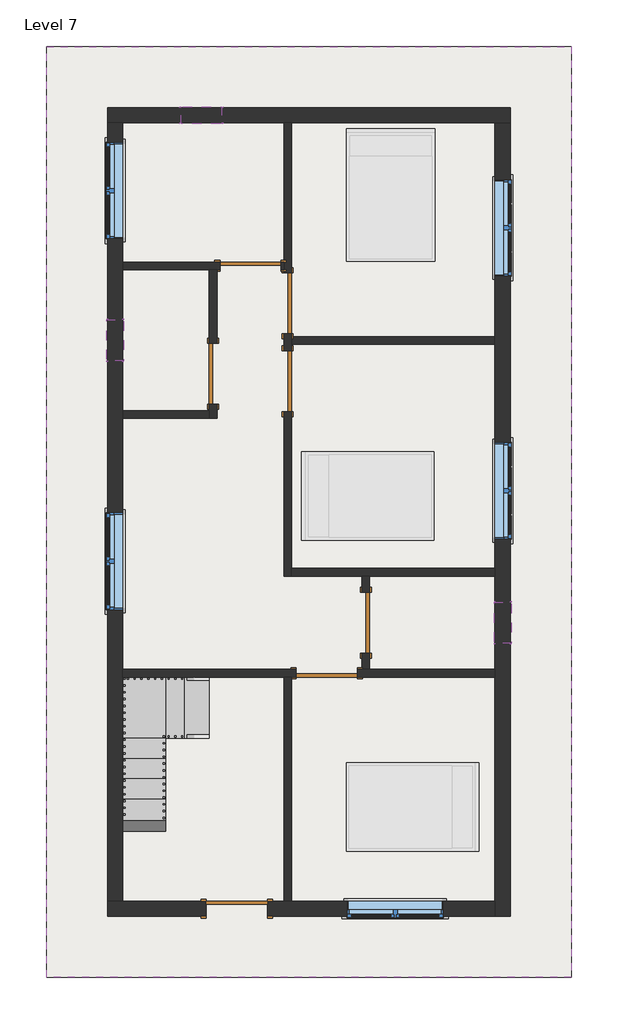
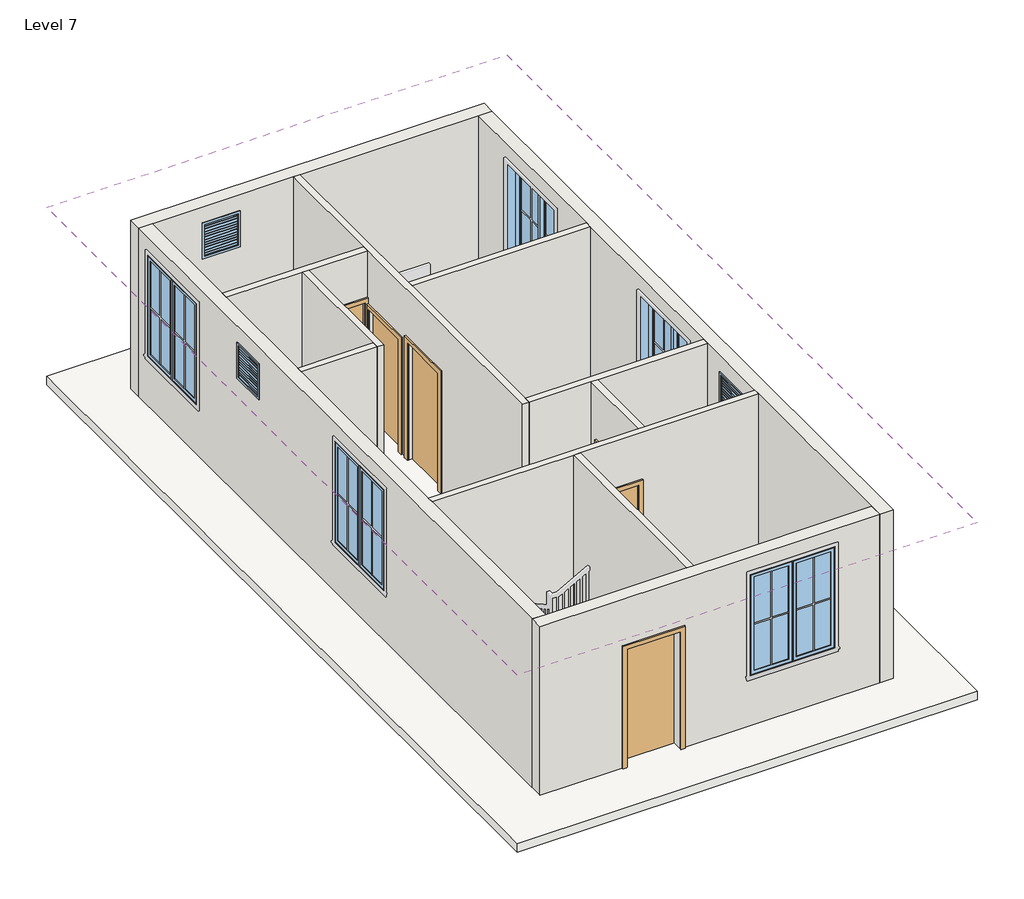
# One storey, part 1 of 2: 13 walls, 8 windows, 7 doors, 2 roofs, 1 stair flight.
"""IFC4 building model written with IfcOpenShell, lengths in millimetres."""

from ifc_helpers import new_model, si_unit, frame, origin, place, context, project, spatial, polyline, outline, extrude, faceted_brep, transform, mapped, element, save
from components import door_5e62189b, door_17d80c48, door_e5f9f3c4, door_305aa2a5, door_0ca8825f, window_9ac97e1a, window_f2d8fef0

model = new_model("IFC4")

# Units and contexts
model_context = context("Model", 3, world=origin())
ifc_project = project(units=[si_unit("LENGTHUNIT", "METRE", prefix="MILLI")], contexts=[model_context])

# Site, building, storey
site = spatial("IfcSite", under=ifc_project)
building = spatial("IfcBuilding", under=site)
storey = spatial("IfcBuildingStorey", under=building, Name="Level 7", Elevation=16002.0)

# Doors
placement = place(None, origin())
door_shape = door_5e62189b(model_context)
element("IfcDoor", 1, ObjectType="Single-Flush : 36\" x 80\"", at=placement, inside=storey, context=model_context, shape_type="MappedRepresentation", body=[
    mapped(door_shape, transform((-2690.3389285, 2204.6069249, 16002.0), x_axis=(0.0, -1.0, 0.0), y_axis=(1.0, 0.0, 0.0), z_axis=(0.0, 0.0, 1.0))),
])
element("IfcDoor", 2, ObjectType="Single-Flush : 36\" x 80\"", at=placement, inside=storey, context=model_context, shape_type="MappedRepresentation", body=[
    mapped(door_shape, transform((-404.3389285, -1522.8430751, 16002.0), x_axis=(0.0, 1.0, 0.0), y_axis=(-1.0, 0.0, 0.0), z_axis=(0.0, 0.0, 1.0))),
])
door_2_shape = door_17d80c48(model_context)
element("IfcDoor", 3, ObjectType="Single-Flush : 36\" x 80\"", at=placement, inside=storey, context=model_context, shape_type="MappedRepresentation", body=[
    mapped(door_2_shape, transform((-1572.7389285, 3258.7069249, 16002.0), x_axis=(0.0, -1.0, 0.0), y_axis=(1.0, 0.0, 0.0), z_axis=(0.0, 0.0, 1.0))),
])
door_3_shape = door_e5f9f3c4(model_context)
element("IfcDoor", 4, ObjectType="Single-Flush : 36\" x 84\"", at=placement, inside=storey, context=model_context, shape_type="MappedRepresentation", body=[
    mapped(door_3_shape, transform((-2131.5389285, 3817.5069249, 16002.0), x_axis=(1.0, 0.0, 0.0), y_axis=(0.0, 1.0, 0.0), z_axis=(0.0, 0.0, 1.0))),
])
element("IfcDoor", 5, ObjectType="Single-Flush : 36\" x 84\"", at=placement, inside=storey, context=model_context, shape_type="MappedRepresentation", body=[
    mapped(door_3_shape, transform((-988.5389285, -2278.4930751, 16002.0), x_axis=(-1.0, 0.0, 0.0), y_axis=(0.0, -1.0, 0.0), z_axis=(0.0, 0.0, 1.0))),
])
door_4_shape = door_305aa2a5(model_context)
element("IfcDoor", 6, ObjectType="Single-Flush : 36\" x 84\"", at=placement, inside=storey, context=model_context, shape_type="MappedRepresentation", body=[
    mapped(door_4_shape, transform((-1572.7389285, 2090.3069249, 16002.0), x_axis=(0.0, 1.0, 0.0), y_axis=(-1.0, 0.0, 0.0), z_axis=(0.0, 0.0, 1.0))),
])
door_5_shape = door_0ca8825f(model_context)
element("IfcDoor", 7, ObjectType="Single-Flush : 36\" x 84\"", at=placement, inside=storey, context=model_context, shape_type="MappedRepresentation", body=[
    mapped(door_5_shape, transform((-2334.7389285, -5802.7430751, 16002.0), x_axis=(1.0, 0.0, 0.0), y_axis=(0.0, 1.0, 0.0), z_axis=(0.0, 0.0, 1.0))),
])

# Roofs
element("IfcRoof", 8, ObjectType="ROOF 6\"", at=placement, inside=storey, context=model_context, shape_type="SweptSolid", body=[
    extrude(outline(polyline([(-5185.8889285, 7100.4569249), (2675.4110715, 7100.4569249), (2675.4110715, -6831.4430751), (-5185.8889285, -6831.4430751), (-5185.8889285, 7100.4569249)])), frame((0.0, 0.0, 15849.6), z_axis=(0.0, 0.0, 1.0), x_axis=(1.0, 0.0, 0.0)), (0.0, 0.0, 1.0), 152.4),
])
element("IfcRoof", 9, ObjectType="ROOF 6\"", at=placement, inside=storey, context=model_context, shape_type="SweptSolid", body=[
    extrude(outline(polyline([(-5185.8889285, 7100.4569249), (2675.4110715, 7100.4569249), (2675.4110715, -6831.4430751), (-5185.8889285, -6831.4430751), (-5185.8889285, 7100.4569249)])), frame((0.0, 0.0, 19050.0), z_axis=(0.0, 0.0, 1.0), x_axis=(1.0, 0.0, 0.0)), (0.0, 0.0, 1.0), 152.4),
])

# Stair flight
element("IfcStairFlight", 10, ObjectType="3/4\" Nosing", at=placement, inside=storey, context=model_context, shape_type="Brep", body=[
    faceted_brep([(-2747.4889285, -3250.0430751, 16171.3333333), (-2747.4889285, -2335.6430751, 16171.3333333), (-3128.4889285, -2335.6430751, 16171.3333333), (-3128.4889285, -3250.0430751, 16171.3333333), (-3128.4889285, -3250.0430751, 16107.8333333), (-2754.6326785, -3250.0430751, 16107.8333333), (-2754.6326785, -2335.6430751, 16107.8333333), (-3128.4889285, -2335.6430751, 16107.8333333)], [[[0, 1, 2, 3]], [[0, 3, 4, 5]], [[2, 1, 6, 7]], [[1, 0, 5, 6]], [[4, 7, 6, 5]], [[7, 4, 3, 2]]]),
    faceted_brep([(-3128.4889285, -3250.0430751, 16340.6666667), (-3128.4889285, -2335.6430751, 16340.6666667), (-3401.5389285, -2335.6430751, 16340.6666667), (-3401.5389285, -3250.0430751, 16340.6666667), (-3401.5389285, -3250.0430751, 16277.1666667), (-3135.6326785, -3250.0430751, 16277.1666667), (-3135.6326785, -2335.6430751, 16277.1666667), (-3401.5389285, -2335.6430751, 16277.1666667)], [[[0, 1, 2, 3]], [[0, 3, 4, 5]], [[2, 1, 6, 7]], [[1, 0, 5, 6]], [[4, 7, 6, 5]], [[7, 4, 3, 2]]]),
    faceted_brep([(-3401.5389285, -3269.0930751, 16510.0), (-3401.5389285, -3250.0430751, 16510.0), (-3401.5389285, -2335.6430751, 16510.0), (-4042.8889285, -2335.6430751, 16510.0), (-4042.8889285, -3269.0930751, 16510.0), (-3401.5389285, -3269.0930751, 16446.5), (-3401.5389285, -3250.0430751, 16446.5), (-3408.6826785, -3250.0430751, 16446.5), (-3408.6826785, -2335.6430751, 16446.5), (-4042.8889285, -2335.6430751, 16446.5), (-4042.8889285, -3269.0930751, 16446.5), (-3401.5389285, -3250.0430751, 16679.3333333), (-4042.8889285, -3250.0430751, 16679.3333333), (-4042.8889285, -3285.5502386, 16679.3333333), (-4042.8889285, -3573.8930751, 16679.3333333), (-3401.5389285, -3573.8930751, 16679.3333333), (-3401.5389285, -3285.5502386, 16679.3333333), (-3401.5389285, -3573.8930751, 16606.7200976), (-3401.5389285, -3285.5502386, 16446.5), (-4042.8889285, -3285.5502386, 16446.5), (-4042.8889285, -3573.8930751, 16606.7200976), (-3401.5389285, -3554.8430751, 16848.6666667), (-4042.8889285, -3554.8430751, 16848.6666667), (-4042.8889285, -3878.6930751, 16848.6666667), (-3401.5389285, -3878.6930751, 16848.6666667), (-3401.5389285, -3878.6930751, 16776.0847552), (-4042.8889285, -3878.6930751, 16776.0847552), (-3401.5389285, -3859.6430751, 17018.0), (-4042.8889285, -3859.6430751, 17018.0), (-4042.8889285, -4183.4930751, 17018.0), (-3401.5389285, -4183.4930751, 17018.0), (-3401.5389285, -4183.4930751, 16945.4494128), (-4042.8889285, -4183.4930751, 16945.4494128), (-3401.5389285, -4164.4430751, 17187.3333333), (-4042.8889285, -4164.4430751, 17187.3333333), (-4042.8889285, -4488.2930751, 17187.3333333), (-3401.5389285, -4488.2930751, 17187.3333333), (-3401.5389285, -4488.2930751, 17114.8140703), (-4042.8889285, -4488.2930751, 17114.8140703), (-3401.5389285, -4792.8112092, 17356.6666667), (-3401.5389285, -4469.2430751, 17356.6666667), (-4042.8889285, -4469.2430751, 17356.6666667), (-4042.8889285, -4792.8112092, 17356.6666667), (-3401.5389285, -4773.7612092, 17526.0), (-3401.5389285, -5114.0119996, 17526.0), (-3401.5389285, -5114.0119996, 17462.5), (-4042.8889285, -4792.8112092, 17284.0221068), (-4042.8889285, -4773.7612092, 17526.0), (-4042.8889285, -5114.0119996, 17526.0), (-4042.8889285, -5688.4430751, 17526.0), (-3401.5389285, -5688.4430751, 17526.0), (-4042.8889285, -5114.0119996, 17462.5), (-4042.8889285, -5688.4430751, 17462.5), (-3401.5389285, -5688.4430751, 17462.5)], [[[0, 1, 2, 3, 4]], [[1, 0, 5, 6]], [[7, 1, 6]], [[3, 2, 8, 9]], [[4, 3, 9, 10]], [[11, 12, 13, 14, 15, 16]], [[0, 11, 16, 15, 17, 18, 5]], [[12, 4, 10, 19, 20, 14, 13]], [[21, 22, 23, 24]], [[21, 24, 25, 17, 15]], [[23, 22, 14, 20, 26]], [[27, 28, 29, 30]], [[27, 30, 31, 25, 24]], [[29, 28, 23, 26, 32]], [[33, 34, 35, 36]], [[33, 36, 37, 31, 30]], [[35, 34, 29, 32, 38]], [[39, 40, 41, 42]], [[39, 43, 44, 45, 37, 36, 40]], [[42, 41, 35, 38, 46]], [[43, 47, 48, 49, 50, 44]], [[47, 42, 46, 51, 52, 49, 48]], [[50, 49, 52, 53]], [[2, 1, 7, 8]], [[0, 4, 12, 11]], [[15, 14, 22, 21]], [[24, 23, 28, 27]], [[30, 29, 34, 33]], [[36, 35, 41, 40]], [[39, 42, 47, 43]], [[18, 19, 10, 9, 8, 7, 6, 5]], [[19, 18, 17, 25, 31, 37, 45, 51, 46, 38, 32, 26, 20]], [[45, 53, 52, 51]], [[53, 45, 44, 50]]]),
    faceted_brep([(-3401.5389285, -4773.7612092, 17695.3333333), (-3401.5389285, -5688.4430751, 17695.3333333), (-3128.4889285, -5688.4430751, 17695.3333333), (-3128.4889285, -4773.7612092, 17695.3333333), (-3394.3951785, -4773.7612092, 17631.8333333), (-3128.4889285, -4773.7612092, 17631.8333333), (-3394.3951785, -5688.4430751, 17631.8333333), (-3128.4889285, -5688.4430751, 17631.8333333)], [[[0, 1, 2, 3]], [[4, 0, 3, 5]], [[2, 1, 6, 7]], [[1, 0, 4, 6]], [[5, 7, 6, 4]], [[7, 5, 3, 2]]]),
    faceted_brep([(-3128.4889285, -4773.7612092, 17864.6666667), (-3128.4889285, -5688.4430751, 17864.6666667), (-2793.6303845, -5688.4430751, 17864.6666667), (-2793.6303845, -4773.7612092, 17864.6666667), (-2793.6303845, -4773.7612092, 17801.1666667), (-3121.3451785, -4773.7612092, 17801.1666667), (-3121.3451785, -5688.4430751, 17801.1666667), (-2793.6303845, -5688.4430751, 17801.1666667)], [[[0, 1, 2, 3]], [[0, 3, 4, 5]], [[2, 1, 6, 7]], [[3, 2, 7, 4]], [[1, 0, 5, 6]], [[6, 5, 4, 7]]]),
])

# Walls
element("IfcWall", 11, ObjectType="WALL 4.5\"", at=placement, inside=storey, context=model_context, shape_type="Brep", body=[
    faceted_brep([(-1629.8889285, 2801.5069249, 18034.0), (-1629.8889285, 2801.5069249, 16002.0), (-1629.8889285, 2547.5069249, 16002.0), (-1629.8889285, 2547.5069249, 18135.6), (-1629.8889285, 1633.1069249, 18135.6), (-1629.8889285, 1633.1069249, 16002.0), (-1629.8889285, -824.3430751, 16002.0), (-1629.8889285, -824.3430751, 19050.0), (-1629.8889285, 3760.3569249, 19050.0), (-1629.8889285, 3874.6569249, 19050.0), (-1629.8889285, 5957.4569249, 19050.0), (-1629.8889285, 5957.4569249, 16002.0), (-1629.8889285, 3874.6569249, 16002.0), (-1629.8889285, 3760.3569249, 16002.0), (-1629.8889285, 3715.9069249, 16002.0), (-1629.8889285, 3715.9069249, 18034.0), (-1515.5889285, 2547.5069249, 16002.0), (-1515.5889285, 2642.7569249, 16002.0), (-1515.5889285, 2757.0569249, 16002.0), (-1515.5889285, 2801.5069249, 16002.0), (-1515.5889285, 2801.5069249, 18034.0), (-1515.5889285, 3715.9069249, 18034.0), (-1515.5889285, 3715.9069249, 16002.0), (-1515.5889285, 5957.4569249, 16002.0), (-1515.5889285, 5957.4569249, 19050.0), (-1515.5889285, 2757.0569249, 19050.0), (-1515.5889285, 2642.7569249, 19050.0), (-1515.5889285, -710.0430751, 19050.0), (-1515.5889285, -824.3430751, 19050.0), (-1515.5889285, -824.3430751, 16002.0), (-1515.5889285, -710.0430751, 16002.0), (-1515.5889285, 1633.1069249, 16002.0), (-1515.5889285, 1633.1069249, 18135.6), (-1515.5889285, 2547.5069249, 18135.6)], [[[0, 1, 2, 3, 4, 5, 6, 7, 8, 9, 10, 11, 12, 13, 14, 15]], [[16, 17, 18, 19, 20, 21, 22, 23, 24, 25, 26, 27, 28, 29, 30, 31, 32, 33]], [[31, 30, 29, 6, 5]], [[2, 1, 19, 18, 17, 16]], [[14, 13, 12, 11, 23, 22]], [[11, 10, 24, 23]], [[3, 2, 16, 33]], [[4, 3, 33, 32]], [[5, 4, 32, 31]], [[20, 19, 1, 0]], [[21, 20, 0, 15]], [[22, 21, 15, 14]], [[10, 9, 8, 7, 28, 27, 26, 25, 24]], [[7, 6, 29, 28]]]),
])
element("IfcWall", 12, ObjectType="WALL 4.5\"", at=placement, inside=storey, context=model_context, shape_type="Brep", body=[
    faceted_brep([(1532.4110715, -710.0430751, 16002.0), (-1515.5889285, -710.0430751, 16002.0), (-1515.5889285, -710.0430751, 19050.0), (1532.4110715, -710.0430751, 19050.0), (1532.4110715, -824.3430751, 16002.0), (1532.4110715, -824.3430751, 19050.0), (-347.1889285, -824.3430751, 19050.0), (-461.4889285, -824.3430751, 19050.0), (-1515.5889285, -824.3430751, 19050.0), (-1515.5889285, -824.3430751, 16002.0), (-461.4889285, -824.3430751, 16002.0), (-347.1889285, -824.3430751, 16002.0)], [[[0, 1, 2, 3]], [[4, 5, 6, 7, 8, 9, 10, 11]], [[1, 0, 4, 11, 10, 9]], [[0, 3, 5, 4]], [[3, 2, 8, 7, 6, 5]], [[2, 1, 9, 8]]]),
])
element("IfcWall", 13, ObjectType="WALL 4.5\"", at=placement, inside=storey, context=model_context, shape_type="SweptSolid", body=[
    extrude(outline(polyline([(-1515.5889285, 2757.0569249), (1532.4110715, 2757.0569249), (1532.4110715, 2642.7569249), (-1515.5889285, 2642.7569249), (-1515.5889285, 2757.0569249)])), frame((0.0, 0.0, 16002.0), z_axis=(0.0, 0.0, 1.0), x_axis=(1.0, 0.0, 0.0)), (0.0, 0.0, 1.0), 3048.0),
])
element("IfcWall", 14, ObjectType="WALL 4.5\"", at=placement, inside=storey, context=model_context, shape_type="Brep", body=[
    faceted_brep([(-1674.3389285, 3760.3569249, 18135.6), (-1674.3389285, 3760.3569249, 16002.0), (-1629.8889285, 3760.3569249, 16002.0), (-1629.8889285, 3760.3569249, 19050.0), (-2633.1889285, 3760.3569249, 19050.0), (-2747.4889285, 3760.3569249, 19050.0), (-4042.8889285, 3760.3569249, 19050.0), (-4042.8889285, 3760.3569249, 16002.0), (-2747.4889285, 3760.3569249, 16002.0), (-2633.1889285, 3760.3569249, 16002.0), (-2588.7389285, 3760.3569249, 16002.0), (-2588.7389285, 3760.3569249, 18135.6), (-1629.8889285, 3874.6569249, 16002.0), (-1674.3389285, 3874.6569249, 16002.0), (-1674.3389285, 3874.6569249, 18135.6), (-2588.7389285, 3874.6569249, 18135.6), (-2588.7389285, 3874.6569249, 16002.0), (-4042.8889285, 3874.6569249, 16002.0), (-4042.8889285, 3874.6569249, 19050.0), (-1629.8889285, 3874.6569249, 19050.0)], [[[0, 1, 2, 3, 4, 5, 6, 7, 8, 9, 10, 11]], [[12, 13, 14, 15, 16, 17, 18, 19]], [[2, 1, 13, 12]], [[10, 9, 8, 7, 17, 16]], [[7, 6, 18, 17]], [[3, 2, 12, 19]], [[14, 13, 1, 0]], [[15, 14, 0, 11]], [[16, 15, 11, 10]], [[6, 5, 4, 3, 19, 18]]]),
])
element("IfcWall", 15, ObjectType="WALL 4.5\"", at=placement, inside=storey, context=model_context, shape_type="Brep", body=[
    faceted_brep([(-2747.4889285, 1747.4069249, 18034.0), (-2747.4889285, 1747.4069249, 16002.0), (-2747.4889285, 1652.1569249, 16002.0), (-2747.4889285, 1537.8569249, 16002.0), (-2747.4889285, 1537.8569249, 19050.0), (-2747.4889285, 1652.1569249, 19050.0), (-2747.4889285, 3760.3569249, 19050.0), (-2747.4889285, 3760.3569249, 16002.0), (-2747.4889285, 2661.8069249, 16002.0), (-2747.4889285, 2661.8069249, 18034.0), (-2633.1889285, 1537.8569249, 16002.0), (-2633.1889285, 1747.4069249, 16002.0), (-2633.1889285, 1747.4069249, 18034.0), (-2633.1889285, 2661.8069249, 18034.0), (-2633.1889285, 2661.8069249, 16002.0), (-2633.1889285, 3760.3569249, 16002.0), (-2633.1889285, 3760.3569249, 19050.0), (-2633.1889285, 1537.8569249, 19050.0)], [[[0, 1, 2, 3, 4, 5, 6, 7, 8, 9]], [[10, 11, 12, 13, 14, 15, 16, 17]], [[8, 7, 15, 14]], [[3, 2, 1, 11, 10]], [[7, 6, 16, 15]], [[4, 3, 10, 17]], [[12, 11, 1, 0]], [[13, 12, 0, 9]], [[14, 13, 9, 8]], [[6, 5, 4, 17, 16]]]),
])
element("IfcWall", 16, ObjectType="WALL 4.5\"", at=placement, inside=storey, context=model_context, shape_type="SweptSolid", body=[
    extrude(outline(polyline([(-4042.8889285, 1652.1569249), (-2747.4889285, 1652.1569249), (-2747.4889285, 1537.8569249), (-4042.8889285, 1537.8569249), (-4042.8889285, 1652.1569249)])), frame((0.0, 0.0, 16002.0), z_axis=(0.0, 0.0, 1.0), x_axis=(1.0, 0.0, 0.0)), (0.0, 0.0, 1.0), 3048.0),
])
element("IfcWall", 17, ObjectType="WALL 4.5\"", at=placement, inside=storey, context=model_context, shape_type="Brep", body=[
    faceted_brep([(-4042.8889285, -2335.6430751, 16002.0), (-1629.8889285, -2335.6430751, 16002.0), (-1515.5889285, -2335.6430751, 16002.0), (-1445.7389285, -2335.6430751, 16002.0), (-1445.7389285, -2335.6430751, 18135.6), (-531.3389285, -2335.6430751, 18135.6), (-531.3389285, -2335.6430751, 16002.0), (1532.4110715, -2335.6430751, 16002.0), (1532.4110715, -2335.6430751, 19050.0), (-1515.5889285, -2335.6430751, 19050.0), (-1629.8889285, -2335.6430751, 19050.0), (-4042.8889285, -2335.6430751, 19050.0), (-1445.7389285, -2221.3430751, 18135.6), (-1445.7389285, -2221.3430751, 16002.0), (-4042.8889285, -2221.3430751, 16002.0), (-4042.8889285, -2221.3430751, 19050.0), (-461.4889285, -2221.3430751, 19050.0), (-347.1889285, -2221.3430751, 19050.0), (1532.4110715, -2221.3430751, 19050.0), (1532.4110715, -2221.3430751, 16002.0), (-347.1889285, -2221.3430751, 16002.0), (-461.4889285, -2221.3430751, 16002.0), (-531.3389285, -2221.3430751, 16002.0), (-531.3389285, -2221.3430751, 18135.6)], [[[0, 1, 2, 3, 4, 5, 6, 7, 8, 9, 10, 11]], [[12, 13, 14, 15, 16, 17, 18, 19, 20, 21, 22, 23]], [[14, 13, 3, 2, 1, 0]], [[22, 21, 20, 19, 7, 6]], [[8, 7, 19, 18]], [[0, 11, 15, 14]], [[4, 3, 13, 12]], [[5, 4, 12, 23]], [[6, 5, 23, 22]], [[11, 10, 9, 8, 18, 17, 16, 15]]]),
])
element("IfcWall", 18, ObjectType="WALL 4.5\"", at=placement, inside=storey, context=model_context, shape_type="SweptSolid", body=[
    extrude(outline(polyline([(-824.3430751, 16002.0), (-1065.6430751, 16002.0), (-1065.6430751, 18034.0), (-1980.0430751, 18034.0), (-1980.0430751, 16002.0), (-2221.3430751, 16002.0), (-2221.3430751, 19050.0), (-824.3430751, 19050.0), (-824.3430751, 16002.0)])), frame((-461.4889285, 0.0, 0.0), z_axis=(1.0, 0.0, 0.0), x_axis=(0.0, 1.0, 0.0)), (0.0, 0.0, 1.0), 114.3),
])
element("IfcWall", 19, ObjectType="WALL 4.5\"", at=placement, inside=storey, context=model_context, shape_type="SweptSolid", body=[
    extrude(outline(polyline([(-1629.8889285, -5688.4430751), (-1629.8889285, -2335.6430751), (-1515.5889285, -2335.6430751), (-1515.5889285, -5688.4430751), (-1629.8889285, -5688.4430751)])), frame((0.0, 0.0, 16002.0), z_axis=(0.0, 0.0, 1.0), x_axis=(1.0, 0.0, 0.0)), (0.0, 0.0, 1.0), 3048.0),
])
element("IfcWall", 20, ObjectType="WALL 9\"", at=placement, inside=storey, context=model_context, shape_type="Brep", body=[
    faceted_brep([(-4271.4889285, 5957.4569249, 16002.0), (-4042.8889285, 5957.4569249, 16002.0), (-1629.8889285, 5957.4569249, 16002.0), (-1515.5889285, 5957.4569249, 16002.0), (1532.4110715, 5957.4569249, 16002.0), (1761.0110715, 5957.4569249, 16002.0), (1761.0110715, 5957.4569249, 19050.0), (1532.4110715, 5957.4569249, 19050.0), (-1515.5889285, 5957.4569249, 19050.0), (-1629.8889285, 5957.4569249, 19050.0), (-4042.8889285, 5957.4569249, 19050.0), (-4271.4889285, 5957.4569249, 19050.0), (-2560.1639285, 5957.4569249, 18745.2), (-2560.1639285, 5957.4569249, 18135.6), (-3169.7639285, 5957.4569249, 18135.6), (-3169.7639285, 5957.4569249, 18745.2), (-4271.4889285, 6186.0569249, 16002.0), (-4271.4889285, 6186.0569249, 19050.0), (1761.0110715, 6186.0569249, 19050.0), (1761.0110715, 6186.0569249, 16002.0), (-2560.1639285, 6186.0569249, 18745.2), (-3169.7639285, 6186.0569249, 18745.2), (-3169.7639285, 6186.0569249, 18135.6), (-2560.1639285, 6186.0569249, 18135.6)], [[[0, 1, 2, 3, 4, 5, 6, 7, 8, 9, 10, 11], [12, 13, 14, 15]], [[16, 17, 18, 19], [20, 21, 22, 23]], [[5, 4, 3, 2, 1, 0, 16, 19]], [[6, 5, 19, 18]], [[0, 11, 17, 16]], [[13, 12, 20, 23]], [[14, 13, 23, 22]], [[15, 14, 22, 21]], [[12, 15, 21, 20]], [[11, 10, 9, 8, 7, 6, 18, 17]]]),
])
element("IfcWall", 21, ObjectType="WALL 9\"", at=placement, inside=storey, context=model_context, shape_type="Brep", body=[
    faceted_brep([(1532.4110715, 5957.4569249, 16002.0), (1532.4110715, 2757.0569249, 16002.0), (1532.4110715, 2642.7569249, 16002.0), (1532.4110715, -710.0430751, 16002.0), (1532.4110715, -824.3430751, 16002.0), (1532.4110715, -2221.3430751, 16002.0), (1532.4110715, -2335.6430751, 16002.0), (1532.4110715, -5688.4430751, 16002.0), (1532.4110715, -5917.0430751, 16002.0), (1532.4110715, -5917.0430751, 19050.0), (1532.4110715, -5688.4430751, 19050.0), (1532.4110715, -2335.6430751, 19050.0), (1532.4110715, -2221.3430751, 19050.0), (1532.4110715, -824.3430751, 19050.0), (1532.4110715, -710.0430751, 19050.0), (1532.4110715, 2642.7569249, 19050.0), (1532.4110715, 2757.0569249, 19050.0), (1532.4110715, 5957.4569249, 19050.0), (1532.4110715, 3661.9319249, 18745.2), (1532.4110715, 3661.9319249, 16916.4), (1532.4110715, 5109.7319249, 16916.4), (1532.4110715, 5109.7319249, 18745.2), (1532.4110715, -271.8930751, 18745.2), (1532.4110715, -271.8930751, 16916.4), (1532.4110715, 1175.9069249, 16916.4), (1532.4110715, 1175.9069249, 18745.2), (1532.4110715, -1827.6430751, 18745.2), (1532.4110715, -1827.6430751, 18135.6), (1532.4110715, -1218.0430751, 18135.6), (1532.4110715, -1218.0430751, 18745.2), (1761.0110715, 5957.4569249, 16002.0), (1761.0110715, 5957.4569249, 19050.0), (1761.0110715, -5917.0430751, 19050.0), (1761.0110715, -5917.0430751, 16002.0), (1761.0110715, 3661.9319249, 18745.2), (1761.0110715, 5109.7319249, 18745.2), (1761.0110715, 5109.7319249, 16916.4), (1761.0110715, 3661.9319249, 16916.4), (1761.0110715, -271.8930751, 18745.2), (1761.0110715, 1175.9069249, 18745.2), (1761.0110715, 1175.9069249, 16916.4), (1761.0110715, -271.8930751, 16916.4), (1761.0110715, -1827.6430751, 18745.2), (1761.0110715, -1218.0430751, 18745.2), (1761.0110715, -1218.0430751, 18135.6), (1761.0110715, -1827.6430751, 18135.6)], [[[0, 1, 2, 3, 4, 5, 6, 7, 8, 9, 10, 11, 12, 13, 14, 15, 16, 17], [18, 19, 20, 21], [22, 23, 24, 25], [26, 27, 28, 29]], [[30, 31, 32, 33], [34, 35, 36, 37], [38, 39, 40, 41], [42, 43, 44, 45]], [[8, 7, 6, 5, 4, 3, 2, 1, 0, 30, 33]], [[0, 17, 31, 30]], [[9, 8, 33, 32]], [[19, 18, 34, 37]], [[20, 19, 37, 36]], [[21, 20, 36, 35]], [[18, 21, 35, 34]], [[23, 22, 38, 41]], [[24, 23, 41, 40]], [[25, 24, 40, 39]], [[22, 25, 39, 38]], [[27, 26, 42, 45]], [[28, 27, 45, 44]], [[29, 28, 44, 43]], [[26, 29, 43, 42]], [[17, 16, 15, 14, 13, 12, 11, 10, 9, 32, 31]]]),
])
element("IfcWall", 22, ObjectType="WALL 9\"", at=placement, inside=storey, context=model_context, shape_type="Brep", body=[
    faceted_brep([(1532.4110715, -5688.4430751, 16002.0), (-1515.5889285, -5688.4430751, 16002.0), (-1629.8889285, -5688.4430751, 16002.0), (-1877.5389285, -5688.4430751, 16002.0), (-1877.5389285, -5688.4430751, 18135.6), (-2791.9389285, -5688.4430751, 18135.6), (-2791.9389285, -5688.4430751, 16002.0), (-4042.8889285, -5688.4430751, 16002.0), (-4271.4889285, -5688.4430751, 16002.0), (-4271.4889285, -5688.4430751, 19050.0), (-4042.8889285, -5688.4430751, 19050.0), (-1629.8889285, -5688.4430751, 19050.0), (-1515.5889285, -5688.4430751, 19050.0), (1532.4110715, -5688.4430751, 19050.0), (-686.9139285, -5688.4430751, 18745.2), (-686.9139285, -5688.4430751, 16916.4), (760.8860715, -5688.4430751, 16916.4), (760.8860715, -5688.4430751, 18745.2), (-1877.5389285, -5917.0430751, 18135.6), (-1877.5389285, -5917.0430751, 16002.0), (1532.4110715, -5917.0430751, 16002.0), (1532.4110715, -5917.0430751, 19050.0), (-4271.4889285, -5917.0430751, 19050.0), (-4271.4889285, -5917.0430751, 16002.0), (-2791.9389285, -5917.0430751, 16002.0), (-2791.9389285, -5917.0430751, 18135.6), (-686.9139285, -5917.0430751, 18745.2), (760.8860715, -5917.0430751, 18745.2), (760.8860715, -5917.0430751, 16916.4), (-686.9139285, -5917.0430751, 16916.4)], [[[0, 1, 2, 3, 4, 5, 6, 7, 8, 9, 10, 11, 12, 13], [14, 15, 16, 17]], [[18, 19, 20, 21, 22, 23, 24, 25], [26, 27, 28, 29]], [[24, 23, 8, 7, 6]], [[20, 19, 3, 2, 1, 0]], [[0, 13, 21, 20]], [[9, 8, 23, 22]], [[15, 14, 26, 29]], [[16, 15, 29, 28]], [[17, 16, 28, 27]], [[14, 17, 27, 26]], [[4, 3, 19, 18]], [[5, 4, 18, 25]], [[6, 5, 25, 24]], [[13, 12, 11, 10, 9, 22, 21]]]),
])
element("IfcWall", 23, ObjectType="WALL 9\"", at=placement, inside=storey, context=model_context, shape_type="Brep", body=[
    faceted_brep([(-4042.8889285, -5688.4430751, 16002.0), (-4042.8889285, -2335.6430751, 16002.0), (-4042.8889285, -2221.3430751, 16002.0), (-4042.8889285, 1537.8569249, 16002.0), (-4042.8889285, 1652.1569249, 16002.0), (-4042.8889285, 3760.3569249, 16002.0), (-4042.8889285, 3874.6569249, 16002.0), (-4042.8889285, 5957.4569249, 16002.0), (-4042.8889285, 5957.4569249, 19050.0), (-4042.8889285, 3874.6569249, 19050.0), (-4042.8889285, 3760.3569249, 19050.0), (-4042.8889285, 1652.1569249, 19050.0), (-4042.8889285, 1537.8569249, 19050.0), (-4042.8889285, -2221.3430751, 19050.0), (-4042.8889285, -2335.6430751, 19050.0), (-4042.8889285, -5688.4430751, 19050.0), (-4042.8889285, 5668.5319249, 18745.2), (-4042.8889285, 5668.5319249, 16916.4), (-4042.8889285, 4220.7319249, 16916.4), (-4042.8889285, 4220.7319249, 18745.2), (-4042.8889285, 121.8069249, 18745.2), (-4042.8889285, 121.8069249, 16916.4), (-4042.8889285, -1325.9930751, 16916.4), (-4042.8889285, -1325.9930751, 18745.2), (-4042.8889285, 2401.4569249, 18745.2), (-4042.8889285, 3011.0569249, 18745.2), (-4042.8889285, 3011.0569249, 18135.6), (-4042.8889285, 2401.4569249, 18135.6), (-4271.4889285, -5688.4430751, 16002.0), (-4271.4889285, -5688.4430751, 19050.0), (-4271.4889285, 5957.4569249, 19050.0), (-4271.4889285, 5957.4569249, 16002.0), (-4271.4889285, 5668.5319249, 18745.2), (-4271.4889285, 4220.7319249, 18745.2), (-4271.4889285, 4220.7319249, 16916.4), (-4271.4889285, 5668.5319249, 16916.4), (-4271.4889285, 121.8069249, 18745.2), (-4271.4889285, -1325.9930751, 18745.2), (-4271.4889285, -1325.9930751, 16916.4), (-4271.4889285, 121.8069249, 16916.4), (-4271.4889285, 2401.4569249, 18745.2), (-4271.4889285, 2401.4569249, 18135.6), (-4271.4889285, 3011.0569249, 18135.6), (-4271.4889285, 3011.0569249, 18745.2)], [[[0, 1, 2, 3, 4, 5, 6, 7, 8, 9, 10, 11, 12, 13, 14, 15], [16, 17, 18, 19], [20, 21, 22, 23], [24, 25, 26, 27]], [[28, 29, 30, 31], [32, 33, 34, 35], [36, 37, 38, 39], [40, 41, 42, 43]], [[7, 6, 5, 4, 3, 2, 1, 0, 28, 31]], [[0, 15, 29, 28]], [[8, 7, 31, 30]], [[17, 16, 32, 35]], [[18, 17, 35, 34]], [[19, 18, 34, 33]], [[16, 19, 33, 32]], [[21, 20, 36, 39]], [[22, 21, 39, 38]], [[23, 22, 38, 37]], [[20, 23, 37, 36]], [[41, 40, 24, 27]], [[42, 41, 27, 26]], [[43, 42, 26, 25]], [[40, 43, 25, 24]], [[15, 14, 13, 12, 11, 10, 9, 8, 30, 29]]]),
])

# Windows
window_shape = window_9ac97e1a(model_context)
element("IfcWindow", 24, ObjectType="Window-Casement-Double : 57\" x 72\"", at=placement, inside=storey, context=model_context, shape_type="MappedRepresentation", body=[
    mapped(window_shape, transform((-4157.1889285, 4944.6319249, 16002.0), x_axis=(0.0, 1.0, 0.0), y_axis=(-1.0, 0.0, 0.0), z_axis=(0.0, 0.0, 1.0))),
])
element("IfcWindow", 25, ObjectType="Window-Casement-Double : 57\" x 72\"", at=placement, inside=storey, context=model_context, shape_type="MappedRepresentation", body=[
    mapped(window_shape, transform((1646.7110715, 4385.8319249, 16002.0), x_axis=(0.0, -1.0, 0.0), y_axis=(1.0, 0.0, 0.0), z_axis=(0.0, 0.0, 1.0))),
])
element("IfcWindow", 26, ObjectType="Window-Casement-Double : 57\" x 72\"", at=placement, inside=storey, context=model_context, shape_type="MappedRepresentation", body=[
    mapped(window_shape, transform((-4157.1889285, -602.0930751, 16002.0), x_axis=(0.0, 1.0, 0.0), y_axis=(-1.0, 0.0, 0.0), z_axis=(0.0, 0.0, 1.0))),
])
element("IfcWindow", 27, ObjectType="Window-Casement-Double : 57\" x 72\"", at=placement, inside=storey, context=model_context, shape_type="MappedRepresentation", body=[
    mapped(window_shape, transform((1646.7110715, 452.0069249, 16002.0), x_axis=(0.0, -1.0, 0.0), y_axis=(1.0, 0.0, 0.0), z_axis=(0.0, 0.0, 1.0))),
])
element("IfcWindow", 28, ObjectType="Window-Casement-Double : 57\" x 72\"", at=placement, inside=storey, context=model_context, shape_type="MappedRepresentation", body=[
    mapped(window_shape, transform((36.9860715, -5802.7430751, 16002.0), x_axis=(-1.0, 0.0, 0.0), y_axis=(0.0, -1.0, 0.0), z_axis=(0.0, 0.0, 1.0))),
])
window_2_shape = window_f2d8fef0(model_context)
element("IfcWindow", 29, ObjectType="Window-Louvers : 24\" x 24\"", at=placement, inside=storey, context=model_context, shape_type="MappedRepresentation", body=[
    mapped(window_2_shape, transform((-2864.9639285, 6065.4069249, 17221.2), x_axis=(-1.0, 0.0, 0.0), y_axis=(0.0, -1.0, 0.0), z_axis=(0.0, 0.0, 1.0))),
])
element("IfcWindow", 30, ObjectType="Window-Louvers : 24\" x 24\"", at=placement, inside=storey, context=model_context, shape_type="MappedRepresentation", body=[
    mapped(window_2_shape, transform((-4163.5389285, 2706.2569249, 17221.2), x_axis=(0.0, 1.0, 0.0), y_axis=(-1.0, 0.0, 0.0), z_axis=(0.0, 0.0, 1.0))),
])
element("IfcWindow", 31, ObjectType="Window-Louvers : 24\" x 24\"", at=placement, inside=storey, context=model_context, shape_type="MappedRepresentation", body=[
    mapped(window_2_shape, transform((1640.3610715, -1522.8430751, 17221.2), x_axis=(0.0, 1.0, 0.0), y_axis=(-1.0, 0.0, 0.0), z_axis=(0.0, 0.0, 1.0))),
])

save(model, "model.ifc")

# Revit data of these elements
# Type "Single-Flush : 36\" x 80\""
#   Type Mark = "6"
#   Construction Type Id = "MDOOR"
#   Assembly Code = "C1020"
#   Analytic Construction = "Metal"
#   Thickness = 0' - 2"
#   Heat Transfer Coefficient (U) = 0.651978 BTU/(h·ft²·°F)
#   Height = 6' - 8"
#   Trim Projection Ext = 0' - 1"
#   Trim Projection Int = 0' - 1"
#   Trim Width = 0' - 3"
#   Width = 3' - 0"
#   Define Thermal Properties by = 1
#   Define Thermal Properties by = 1
#   Door Material = Door - Panel
#   Frame Material = Door - Frame
#   Visual Light Transmittance = 0
#   Solar Heat Gain Coefficient = 0
#   Function = (empty or 0)
#   Wall Closure = (empty or 0)
# Type "Single-Flush : 36\" x 84\""
#   Type Mark = "1"
#   Construction Type Id = "MDOOR"
#   Assembly Code = "C1020"
#   Analytic Construction = "Metal"
#   Thickness = 0' - 2"
#   Heat Transfer Coefficient (U) = 0.651978 BTU/(h·ft²·°F)
#   Height = 7' - 0"
#   Trim Projection Ext = 0' - 1"
#   Trim Projection Int = 0' - 1"
#   Trim Width = 0' - 3"
#   Width = 3' - 0"
#   Define Thermal Properties by = 1
#   Define Thermal Properties by = 1
#   Door Material = Door - Panel
#   Frame Material = Door - Frame
#   Visual Light Transmittance = 0
#   Solar Heat Gain Coefficient = 0
#   Function = (empty or 0)
#   Wall Closure = (empty or 0)
# Type "ROOF 6\""
#   Assembly Code = "B1020"
#   Layers, outside or top first: 0' - 6" no material (function 1)
# Type "WALL 4.5\""
#   Assembly Code = "B2010"
#   Layers, outside or top first: 0' - 4 1/2" no material (function 1)
# Type "WALL 9\""
#   Assembly Code = "B2010"
#   Layers, outside or top first: 0' - 9" no material (function 1)
# Type "Window-Casement-Double : 57\" x 72\""
#   Type Mark = "17"
#   Fire Rating = "0.5h"
#   Assembly Code = "B2020100"
#   Analytic Construction = "Double glazing - domestic"
#   Frame Extension [instance default] = 0' - 0 1/4"
#   Window Inset [instance default] = 0' - 0"
#   Wall Thickness [instance default] = 0' - 6"
#   Interior Wall Closure [instance default] = 0' - 2 1/4"
#   Half Width = 2' - 4 1/2"
#   Visual Light Transmittance = 0.81
#   Thermal Resistance (R) = 1.8146 (h·ft²·°F)/BTU
#   Solar Heat Gain Coefficient = 0.76
#   Rough Width = 4' - 9 1/2"
#   Rough Height = 6' - 0 1/2"
#   Height = 6' - 0"
#   Heat Transfer Coefficient (U) = 0.5511 BTU/(h·ft²·°F)
#   Exterior Wall Closure [instance default] = 0' - 1 1/4"
#   Extension Jamb [instance default] = 0' - 2 1/4"
#   Default Sill Height = 3' - 0"
#   Width = 4' - 9"
#   Define Thermal Properties by = 0
#   Muntin Visibility = yes
#   Interior Trim Visibility [instance default] = yes
#   Exterior Trim Visibility [instance default] = yes
#   Extension Jamb Visibility [instance default] = yes
#   Interior Trim Material = Wood - Stained
#   Muntin Pattern = Muntin Pattern_2x2 : Muntin Pattern_2x2
#   Interior Trim = Trim-Window-Interior-Flat : Picture Frame
#   Interior Frame Material = Wood - Stained
#   Glass Panel Material = Glass
#   Exterior Trim Material = Clad - White
#   Exterior Trim = Trim-Window-Exterior-Flat : with Sill
#   Exterior Frame Material = Clad - White
#   Wall Closure = (empty or 0)
# Type "Window-Louvers : 24\" x 24\""
#   Type Mark = "18"
#   Construction Type Id = "GSP4R"
#   Assembly Code = "B20"
#   Analytic Construction = "1/8 in Pilkington single glazing"
#   Visual Light Transmittance = 0.9
#   Thermal Resistance (R) = 1.53941 (h·ft²·°F)/BTU
#   Solar Heat Gain Coefficient = 0.78
#   Max Height = 1' - 11.74264"
#   Height = 2' - 0"
#   Heat Transfer Coefficient (U) = 0.6496 BTU/(h·ft²·°F)
#   Blade Width [instance default] = 1' - 10 1/2"
#   Blade Vertical Thickness = 0' - 0.35355"
#   Blade Thickness = 0' - 0 1/4"
#   Blade Spacing = 0' - 1 1/2"
#   Blade Height = 0' - 1.85355"
#   Blade Depth = 0' - 3"
#   Blade Angle = 45.00°
#   Default Sill Height = 3' - 0"
#   Trim Projection_Exterior = 0' - 0 1/2"
#   Trim Projection_Interior = 0' - 0 1/2"
#   Trim Width_Exterior = 0' - 1 1/2"
#   Trim Width_Interior = 0' - 1 1/2"
#   Width = 2' - 0"
#   Max Blade Count = 12
#   Define Thermal Properties by = 1
#   Blade Count = 12
#   Frame Material = Birch
#   Louver Material = Birch
#   Trim Exterior Material = Birch
#   Trim Interior Material = Birch
#   Wall Closure = (empty or 0)
# Elements 1, 2, 3 (IfcDoor, "Single-Flush : 36\" x 80\"")
#   Phase Created = New Construction
#   Materials on its faces: "Door - Frame", "Door - Panel"
# Elements 4, 5, 6, 7 (IfcDoor, "Single-Flush : 36\" x 84\"")
#   Phase Created = New Construction
#   Materials on its faces: "Door - Frame", "Door - Panel"
# Element 8 (IfcRoof, "ROOF 6\"")
#   built-in parameter 1001705 = 52.5 (stored number, unit not read)
#   built-in parameter 1001701 = -0.5 (stored number, unit not read)
#   built-in parameter 1001710 = 33615
#   Phase Created = New Construction
#   Materials on its faces: "Default Roof", "Door - Panel"
# Element 9 (IfcRoof, "ROOF 6\"")
#   built-in parameter 1001705 = 63 (stored number, unit not read)
#   built-in parameter 1001701 = 10 (stored number, unit not read)
#   built-in parameter 1001710 = 33615
#   Phase Created = New Construction
#   Materials on its faces: "Default Roof", "Door - Panel"
# Element 10 (IfcStairFlight, "3/4\" Nosing")
#   Phase Created = New Construction
#   Materials on its faces: "Concrete, Cast-in-Place gray"
# Elements 11, 12, 13, 14, 15, 16, 17, 18, 19 (IfcWall, "WALL 4.5\"")
#   Top Offset = 0' - 0"
#   Base Offset = 0' - 0"
#   Unconnected Height = 10' - 0"
#   wall height = 10' - 0"
#   Phase Created = New Construction
#   Base Constraint = Level 7
#   Materials on its faces: "Default Wall"
# Elements 20, 21, 22, 23 (IfcWall, "WALL 9\"")
#   Top Offset = 0' - 0"
#   Base Offset = 0' - 0"
#   Unconnected Height = 10' - 0"
#   wall height = 10' - 0"
#   Phase Created = New Construction
#   Base Constraint = Level 7
#   Materials on its faces: "Default Wall", "Copper"
# Element 24 (IfcWindow, "Window-Casement-Double : 57\" x 72\"")
#   Mark = "41"
#   Window Inset = 0' - 0"
#   Interior Wall Closure = 0' - 2 1/4"
#   Frame Extension = 0' - 0 1/4"
#   Exterior Wall Closure = 0' - 1 1/4"
#   Interior Trim Visibility = yes
#   Exterior Trim Visibility = yes
#   Phase Created = New Construction
#   Materials on its faces: "Wood - Stained", "Glass", "Clad - White"
# Element 25 (IfcWindow, "Window-Casement-Double : 57\" x 72\"")
#   Mark = "42"
#   Window Inset = 0' - 0"
#   Interior Wall Closure = 0' - 2 1/4"
#   Frame Extension = 0' - 0 1/4"
#   Exterior Wall Closure = 0' - 1 1/4"
#   Interior Trim Visibility = yes
#   Exterior Trim Visibility = yes
#   Phase Created = New Construction
#   Materials on its faces: "Wood - Stained", "Glass", "Clad - White"
# Element 26 (IfcWindow, "Window-Casement-Double : 57\" x 72\"")
#   Mark = "43"
#   Window Inset = 0' - 0"
#   Interior Wall Closure = 0' - 2 1/4"
#   Frame Extension = 0' - 0 1/4"
#   Exterior Wall Closure = 0' - 1 1/4"
#   Interior Trim Visibility = yes
#   Exterior Trim Visibility = yes
#   Phase Created = New Construction
#   Materials on its faces: "Wood - Stained", "Glass", "Clad - White"
# Element 27 (IfcWindow, "Window-Casement-Double : 57\" x 72\"")
#   Mark = "44"
#   Window Inset = 0' - 0"
#   Interior Wall Closure = 0' - 2 1/4"
#   Frame Extension = 0' - 0 1/4"
#   Exterior Wall Closure = 0' - 1 1/4"
#   Interior Trim Visibility = yes
#   Exterior Trim Visibility = yes
#   Phase Created = New Construction
#   Materials on its faces: "Wood - Stained", "Glass", "Clad - White"
# Element 28 (IfcWindow, "Window-Casement-Double : 57\" x 72\"")
#   Mark = "45"
#   Window Inset = 0' - 0"
#   Interior Wall Closure = 0' - 2 1/4"
#   Frame Extension = 0' - 0 1/4"
#   Exterior Wall Closure = 0' - 1 1/4"
#   Interior Trim Visibility = yes
#   Exterior Trim Visibility = yes
#   Phase Created = New Construction
#   Materials on its faces: "Wood - Stained", "Glass", "Clad - White"
# Element 29 (IfcWindow, "Window-Louvers : 24\" x 24\"")
#   Mark = "46"
#   Blade Width = 1' - 10 1/2"
#   Phase Created = New Construction
#   Materials on its faces: "Birch"
# Element 30 (IfcWindow, "Window-Louvers : 24\" x 24\"")
#   Mark = "47"
#   Blade Width = 1' - 10 1/2"
#   Phase Created = New Construction
#   Materials on its faces: "Birch"
# Element 31 (IfcWindow, "Window-Louvers : 24\" x 24\"")
#   Mark = "48"
#   Blade Width = 1' - 10 1/2"
#   Phase Created = New Construction
#   Materials on its faces: "Birch"
# Materials
#   "Door - Panel": class "Wood", colour RGB 210 159 95, transparency 0, Cost = 0
#   "Door - Frame": colour RGB 118 70 51, transparency 0, Cost = 0
#   "Wood - Stained": class "Wood", colour RGB 224 178 126, transparency 0, Cost = 0
#   "Glass": class "Glass", colour RGB 0 128 192, transparency 0.75, Description = "Soda Lime Glass", Cost = 0
#   "Clad - White": class "Wood", colour RGB 242 242 238, transparency 0, Cost = 0
#   "Birch": class "Wood", colour RGB 224 178 126, transparency 0, Description = "Betula Alleghaniensis", Cost = 0
#   "Default Roof": colour RGB 88 101 114, transparency 0, Cost = 0
#   "Concrete, Cast-in-Place gray": class "Concrete", colour RGB 192 192 192, transparency 0, Description = "Cast-in-place concrete", Cost = 0
#   "Default Wall": colour RGB 128 128 128, transparency 0, Cost = 0
#   "Copper": class "Metal", colour RGB 0 0 0, transparency 0, Description = "Copper, matte finish", Cost = 0
